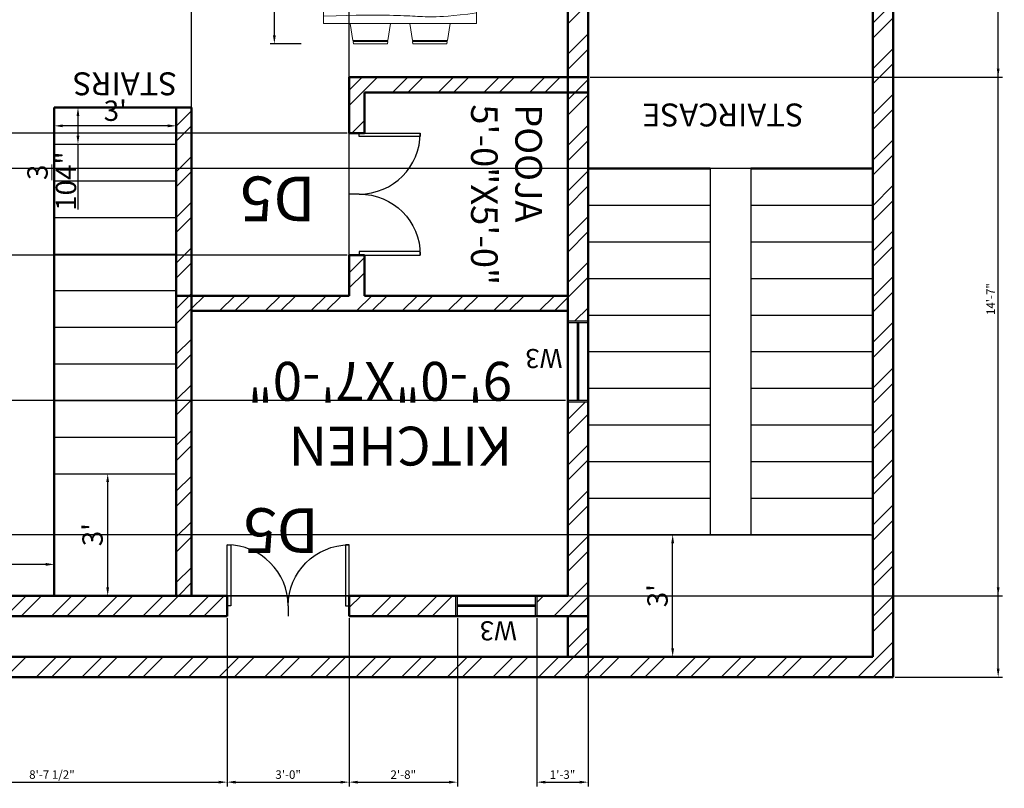
# Model space of a CAD drawing. Units: inches. Extents: x 244 to 2800, y 1060 to 1700.
# Tile 7 of 13: x 1735 to 2025, y 1060 to 1287. Entities that reach past the tile are written whole.
import ezdxf

# ---------------------------------------------------------------- set-up
doc = ezdxf.new("R2010")
doc.units = ezdxf.units.IN
for name, color, linetype, lineweight in [('A-ANNO-DIMS', 2, 'Continuous', 18), ('A-ANNO-TEXT', 1, 'Continuous', 18), ('A-DOOR', 5, 'Continuous', 25), ('A-FLOR-STRS', 6, 'Continuous', 25), ('A-FURN', 9, 'Continuous', 18), ('A-GLAZ', 3, 'Continuous', 25), ('A-WALL', 7, 'Continuous', 50), ('A-WALL-PATT', 8, 'Continuous', 13)]:
    doc.layers.add(name, color=color, linetype=linetype, lineweight=lineweight)
doc.styles.get("Standard").update_dxf_attribs({"font": 'arial.ttf'})
doc.dimstyles.new('ISO-25', dxfattribs={"dimtxt": 2.5, "dimasz": 2.5, "dimexe": 1.25, "dimexo": 0.625, "dimtad": 1, "dimlunit": 4, "dimtxsty": 'Standard', "dimcen": 2.5, "dimadec": 0, "dimazin": 0, "dimtfac": 1, "dimtmove": 0, "dimatfit": 3, "dimfxl": 1, "dimarcsym": 0})

# ---------------------------------------------------------------- blocks, each defined once
blk = doc.blocks.new('*U2')
for p, q in [((0, 0), (0, -5)), ((30, 0), (30, -5))]:
    blk.add_line(p, q)
blk.add_lwpolyline([(0, 0), (0, 30), (1.75, 30), (1.75, 0)], close=True)
blk.add_arc((0, 0), 30, 0, 90)
blk = doc.blocks.new('Dining Set - 36 x 72 in.')
for p, q in [((-22.2343, 26.00059), (-23.4847, 17.99762)), ((-22.2304, 26), (-5.7608, 26)), ((-22, 27.5), (-22.1562, 26.50042)), ((-5.8416, 26.5), (-22.1534, 26.5)), ((-22, 27.5), (-6, 27.5)), ((-5.8437, 26.49966), (-6, 27.5)), ((-4.5152, 17.99762), (-5.7655, 25.99926)), ((5.7657, 26.00059), (4.5153, 17.99762)), ((5.7696, 26), (22.2392, 26)), ((6, 27.5), (5.8438, 26.50042)), ((22.1584, 26.5), (5.8466, 26.5)), ((6, 27.5), (22, 27.5)), ((22.1563, 26.49966), (22, 27.5)), ((23.4848, 17.99762), (22.2345, 25.99926)), ((36, 18), (-36, 18)), ((-36, 18), (-36, -18)), ((36, -18), (36, 18)), ((-44.0006, 8.23428), (-35.9976, 9.48474)), ((44.0006, 8.23428), (35.9976, 9.48474)), ((-45.5, 8), (-44.5004, 8.15617)), ((-45.5, 8), (-45.5, -8)), ((-44.5, -8.15843), (-44.5, 8.15338)), ((-44, 8.23041), (-44, -8.23915)), ((44, 8.23041), (44, -8.23915)), ((44.5, -8.15843), (44.5, 8.15338)), ((45.5, 8), (44.5005, 8.15617)), ((45.5, 8), (45.5, -8)), ((-44.4997, -8.15631), (-45.5, -8)), ((-35.9976, -9.48476), (-43.9993, -8.2345)), ((35.9976, -9.48476), (43.9993, -8.2345)), ((44.4997, -8.15631), (45.5, -8)), ((-36, -18), (36, -18)), ((-22.2343, -26.0006), (-23.4847, -17.99762)), ((-4.5152, -17.99762), (-5.7655, -25.99928)), ((5.7657, -26.0006), (4.5153, -17.99762)), ((23.4848, -17.99762), (22.2345, -25.99928)), ((-22.2304, -26), (-5.7608, -26)), ((-22, -27.5), (-22.1562, -26.50044)), ((-5.8416, -26.5), (-22.1534, -26.5)), ((-22, -27.5), (-6, -27.5)), ((-5.8437, -26.49967), (-6, -27.5)), ((5.7696, -26), (22.2392, -26)), ((6, -27.5), (5.8438, -26.50044)), ((22.1584, -26.5), (5.8466, -26.5)), ((6, -27.5), (22, -27.5)), ((22.1563, -26.49967), (22, -27.5))]:
    blk.add_line(p, q)
for points in [[(-36, 15), (-31.1772, 14.97754), (-26.8079, 14.91406), (-22.8538, 14.81543), (-19.276, 14.6875), (-16.0362, 14.53613), (-13.0957, 14.36718), (-10.4159, 14.18652), (-7.9583, 14), (-5.6904, 13.81315), (-3.6035, 13.63021), (-1.6954, 13.45508), (0.0365, 13.29166), (1.5945, 13.14388), (2.9811, 13.01562), (4.1988, 12.9108), (5.25, 12.83333), (6.1393, 12.78613), (6.8802, 12.76823), (7.4883, 12.77767), (7.9792, 12.8125), (8.3685, 12.87077), (8.6719, 12.95052), (8.9049, 13.0498), (9.0833, 13.16666), (9.2205, 13.29899), (9.3216, 13.44401), (9.3895, 13.59879), (9.4271, 13.76041), (9.4373, 13.92594), (9.4232, 14.09245), (9.3875, 14.257), (9.3333, 14.41666), (9.2638, 14.56917), (9.1836, 14.71484), (9.0975, 14.85465), (9.0104, 14.98958), (8.9272, 15.1206), (8.8529, 15.2487), (8.7922, 15.37483), (8.75, 15.5), (8.7305, 15.62467), (8.7344, 15.74739), (8.7617, 15.86621), (8.8125, 15.97916), (8.8867, 16.08431), (8.9844, 16.17968), (9.1055, 16.26334), (9.25, 16.33333), (9.4189, 16.38802), (9.6172, 16.42708), (9.8506, 16.45052), (10.125, 16.45833), (10.4463, 16.45052), (10.8203, 16.42708), (11.2529, 16.38802), (11.75, 16.33333), (12.3184, 16.26318), (12.9694, 16.17838), (13.7151, 16.07991), (14.5677, 15.96875), (15.5395, 15.84586), (16.6426, 15.71224), (17.8893, 15.56884), (19.2917, 15.41666), (20.859, 15.25667), (22.5879, 15.08984), (24.4721, 14.91715), (26.5052, 14.73958), (28.6809, 14.5581), (30.9929, 14.3737), (33.4347, 14.18733), (36, 14)], [(-36, 10), (-28.9766, 10.14274), (-23.1725, 10.20442), (-18.4241, 10.19775), (-14.5677, 10.13541), (-11.4399, 10.03011), (-8.877, 9.89453), (-6.7154, 9.74137), (-4.7917, 9.58333), (-2.9698, 9.43082), (-1.2246, 9.28515), (0.4415, 9.14534), (2.026, 9.01041), (3.5266, 8.87939), (4.9408, 8.7513), (6.266, 8.62516), (7.5, 8.5), (8.6411, 8.37549), (9.6914, 8.2539), (10.6538, 8.13818), (11.5312, 8.03125), (12.3267, 7.93603), (13.043, 7.85547), (13.6831, 7.79248), (14.25, 7.75), (14.7471, 7.7303), (15.1797, 7.73307), (15.5537, 7.75732), (15.875, 7.80208), (16.1494, 7.86637), (16.3828, 7.94922), (16.5811, 8.04964), (16.75, 8.16666), (16.8944, 8.29915), (17.0143, 8.44531), (17.1089, 8.60319), (17.1771, 8.77083), (17.218, 8.94629), (17.2305, 9.1276), (17.2137, 9.31282), (17.1667, 9.5), (17.0895, 9.6875), (16.987, 9.875), (16.8649, 10.0625), (16.7292, 10.25), (16.5856, 10.4375), (16.4401, 10.625), (16.2985, 10.8125), (16.1667, 11), (16.05, 11.18733), (15.9518, 11.3737), (15.8752, 11.5581), (15.8229, 11.73958), (15.798, 11.91715), (15.8034, 12.08984), (15.842, 12.25667), (15.9167, 12.41666), (16.0295, 12.56836), (16.1784, 12.70833), (16.3605, 12.83268), (16.5729, 12.9375), (16.8127, 13.01888), (17.0768, 13.07291), (17.3625, 13.0957), (17.6667, 13.08333), (17.9894, 13.03312), (18.3418, 12.94726), (18.7382, 12.82918), (19.1927, 12.68229), (19.7195, 12.51001), (20.3327, 12.31575), (21.0465, 12.10294), (21.875, 11.875), (22.8357, 11.63354), (23.959, 11.37304), (25.2786, 11.08618), (26.8282, 10.76562), (28.6414, 10.40405), (30.752, 9.99414), (33.1936, 9.52856), (36, 9)], [(-36, 5.5), (-30.7157, 5.3348), (-26.069, 5.20963), (-21.9946, 5.11767), (-18.4271, 5.05208), (-15.3009, 5.00602), (-12.5508, 4.97265), (-10.1112, 4.94515), (-7.9167, 4.91666), (-5.909, 4.88167), (-4.0586, 4.83984), (-2.3429, 4.79215), (-0.7396, 4.73958), (0.7739, 4.6831), (2.22, 4.6237), (3.6213, 4.56233), (5, 4.5), (6.373, 4.43782), (7.7344, 4.3776), (9.0723, 4.32129), (10.375, 4.27083), (11.6309, 4.22819), (12.8281, 4.19531), (13.9551, 4.17415), (15, 4.16666), (15.954, 4.17448), (16.819, 4.19791), (17.6001, 4.23698), (18.3021, 4.29166), (18.9299, 4.36198), (19.4883, 4.44791), (19.9823, 4.54948), (20.4167, 4.66666), (20.7969, 4.79899), (21.1302, 4.94401), (21.4245, 5.09879), (21.6875, 5.26041), (21.9271, 5.42594), (22.1511, 5.59245), (22.3672, 5.757), (22.5834, 5.91666), (22.8065, 6.06868), (23.0404, 6.21093), (23.2879, 6.34147), (23.5521, 6.45833), (23.8358, 6.55957), (24.142, 6.64323), (24.4735, 6.70735), (24.8334, 6.75), (25.2235, 6.76969), (25.642, 6.76692), (26.0858, 6.74267), (26.5521, 6.69791), (27.0379, 6.63362), (27.5404, 6.55078), (28.0565, 6.45036), (28.5834, 6.33333), (29.1242, 6.19987), (29.7071, 6.04687), (30.3661, 5.87044), (31.1354, 5.66666), (32.0493, 5.43164), (33.142, 5.16146), (34.4475, 4.85221), (36, 4.5)], [(-36, -1), (-30.7915, -0.6591), (-26.0195, -0.38216), (-21.6519, -0.16284), (-17.6563, 0.00521), (-14.0005, 0.12833), (-10.6523, 0.21289), (-7.5796, 0.26522), (-4.75, 0.29166), (-2.134, 0.29793), (0.2878, 0.28711), (2.5317, 0.26163), (4.6146, 0.22396), (6.5529, 0.17651), (8.3633, 0.12174), (10.0623, 0.06209), (11.6667, 0), (13.1899, -0.06201), (14.6341, -0.1211), (15.9982, -0.17432), (17.2813, -0.21875), (18.4823, -0.25147), (19.6003, -0.26953), (20.6343, -0.27002), (21.5834, -0.25), (22.4481, -0.20768), (23.2357, -0.14584), (23.9549, -0.06836), (24.6146, 0.02083), (25.2235, 0.11784), (25.7904, 0.21875), (26.3241, 0.31966), (26.8334, 0.41666), (27.3265, 0.50618), (27.8099, 0.58593), (28.2894, 0.65397), (28.7709, 0.70833), (29.2601, 0.74707), (29.763, 0.76823), (30.2855, 0.76985), (30.8334, 0.75), (31.4088, 0.70784), (31.9994, 0.64713), (32.589, 0.57275), (33.1615, 0.48958), (33.7008, 0.4025), (34.1908, 0.3164), (34.6153, 0.23616), (34.9584, 0.16666), (35.2099, 0.11165), (35.3848, 0.07031), (35.504, 0.04069), (35.5886, 0.02083), (35.6594, 0.00879), (35.7377, 0.0026), (35.8442, 0.00032), (36, 0)], [(-36, -6.5), (-27.1843, -6.31267), (-20.084, -6.1263), (-14.469, -5.9419), (-10.1094, -5.76042), (-6.7752, -5.58285), (-4.2363, -5.41016), (-2.2629, -5.24333), (-0.625, -5.08334), (0.8708, -4.93099), (2.2715, -4.78646), (3.5872, -4.64974), (4.8281, -4.52084), (6.0046, -4.39974), (7.127, -4.28646), (8.2053, -4.18099), (9.25, -4.08334), (10.2705, -3.99382), (11.2734, -3.91407), (12.2647, -3.84603), (13.25, -3.79167), (14.2354, -3.75293), (15.2266, -3.73177), (16.2295, -3.73015), (17.25, -3.75), (18.2912, -3.79248), (19.3451, -3.85547), (20.4009, -3.93604), (21.4479, -4.03125), (22.4754, -4.13819), (23.4727, -4.25391), (24.4289, -4.37549), (25.3334, -4.5), (26.1785, -4.62492), (26.9694, -4.74935), (27.7145, -4.87281), (28.4219, -4.99479), (29.1, -5.11483), (29.7572, -5.23242), (30.4016, -5.34709), (31.0417, -5.45834), (31.6837, -5.56437), (32.3262, -5.65821), (32.9658, -5.73153), (33.599, -5.77604), (34.2224, -5.78345), (34.8327, -5.74545), (35.4264, -5.65373), (36, -5.5)], [(-36, -10), (-26.4022, -9.81299), (-18.4675, -9.62891), (-11.9839, -9.45069), (-6.7396, -9.28125), (-2.5226, -9.12354), (0.8789, -8.98047), (3.6769, -8.85498), (6.0833, -8.75), (8.2767, -8.66765), (10.3021, -8.60677), (12.1712, -8.56543), (13.8958, -8.54167), (15.4876, -8.53353), (16.9583, -8.53907), (18.3197, -8.55632), (19.5834, -8.58334), (20.7616, -8.61841), (21.8685, -8.66081), (22.9188, -8.71004), (23.9271, -8.76563), (24.9081, -8.82707), (25.8763, -8.89388), (26.8465, -8.96558), (27.8334, -9.04167), (28.8474, -9.12118), (29.8828, -9.20117), (30.93, -9.27824), (31.9792, -9.34896), (33.0205, -9.40991), (34.0443, -9.45768), (35.0407, -9.48885), (36, -9.5)], [(-36, -14.5), (-30.0881, -14.33513), (-25.0332, -14.21224), (-20.7312, -14.12647), (-17.0781, -14.07292), (-13.97, -14.04671), (-11.3027, -14.04297), (-8.9724, -14.05681), (-6.875, -14.08334), (-4.9224, -14.11833), (-3.0905, -14.16016), (-1.3709, -14.20785), (0.2448, -14.26042), (1.7647, -14.3169), (3.1973, -14.3763), (4.5507, -14.43767), (5.8333, -14.5), (7.0554, -14.5621), (8.235, -14.62175), (9.3922, -14.67652), (10.5469, -14.72396), (11.7192, -14.76164), (12.929, -14.78711), (14.1965, -14.79794), (15.5417, -14.79167), (16.9933, -14.76424), (18.6152, -14.70508), (20.4804, -14.60197), (22.6615, -14.44271), (25.2312, -14.21509), (28.2624, -13.9069), (31.8277, -13.50594), (36, -13)]]:
    blk.add_lwpolyline(points)
blk = doc.blocks.new('*D38')
at = {"layer": 'A-ANNO-DIMS', "color": 0, "lineweight": -2, "transparency": 16777216}
for p, q in [((1708.9, 1124.22), (1708.9, 1127.48)), ((1744.9, 1124.22), (1744.9, 1127.48)), ((1742.4, 1126.23), (1711.4, 1126.23))]:
    blk.add_line(p, q, dxfattribs=at)
at = {"layer": 'A-ANNO-DIMS', "color": 0, "transparency": 16777216}
for points in [[(1711.4, 1126.65), (1711.4, 1125.81), (1708.9, 1126.23)], [(1742.4, 1126.65), (1742.4, 1125.81), (1744.9, 1126.23)]]:
    blk.add_solid(points, dxfattribs=at)
at = {"layer": 'Defpoints', "color": 0, "transparency": 16777216}
for p in [(1708.9, 1126.23), (1708.9, 1123.59), (1744.9, 1123.59)]:
    blk.add_point(p, dxfattribs=at)
at = {"layer": 'A-ANNO-DIMS', "color": 0, "transparency": 16777216, "insert": (1726.9, 1129.92), "char_height": 6, "attachment_point": 5}
blk.add_mtext("3'", dxfattribs=at)
blk = doc.blocks.new('*D40')
at = {"layer": 'A-ANNO-DIMS', "color": 0, "lineweight": -2, "transparency": 16777216}
for p, q in [((1744.9, 1260.36), (1744.9, 1254.35)), ((1780.9, 1260.36), (1780.9, 1254.35)), ((1778.4, 1255.6), (1747.4, 1255.6))]:
    blk.add_line(p, q, dxfattribs=at)
at = {"layer": 'A-ANNO-DIMS', "color": 0, "transparency": 16777216}
for points in [[(1747.4, 1256.02), (1747.4, 1255.19), (1744.9, 1255.6)], [(1778.4, 1256.02), (1778.4, 1255.19), (1780.9, 1255.6)]]:
    blk.add_solid(points, dxfattribs=at)
at = {"layer": 'Defpoints', "color": 0, "transparency": 16777216}
for p in [(1744.9, 1260.99), (1780.9, 1260.99), (1744.9, 1255.6)]:
    blk.add_point(p, dxfattribs=at)
at = {"layer": 'A-ANNO-DIMS', "color": 0, "transparency": 16777216, "insert": (1762.9, 1259.29), "char_height": 6, "attachment_point": 5}
blk.add_mtext("3'", dxfattribs=at)
blk = doc.blocks.new('*D41')
at = {"layer": 'A-ANNO-DIMS', "color": 0, "lineweight": -2, "transparency": 16777216}
for p, q in [((1745.52, 1260.99), (1753.14, 1260.99)), ((1751.89, 1258.49), (1751.89, 1252.69)), ((1745.52, 1250.19), (1753.14, 1250.19)), ((1751.89, 1250.19), (1751.89, 1230.89))]:
    blk.add_line(p, q, dxfattribs=at)
at = {"layer": 'A-ANNO-DIMS', "color": 0, "transparency": 16777216}
for points in [[(1751.47, 1258.49), (1752.3, 1258.49), (1751.89, 1260.99)], [(1751.47, 1252.69), (1752.3, 1252.69), (1751.89, 1250.19)]]:
    blk.add_solid(points, dxfattribs=at)
at = {"layer": 'Defpoints', "color": 0, "transparency": 16777216}
for p in [(1744.9, 1260.99), (1744.9, 1250.19), (1751.89, 1250.19)]:
    blk.add_point(p, dxfattribs=at)
at = {"layer": 'A-ANNO-DIMS', "color": 0, "transparency": 16777216, "insert": (1744.15, 1239.29), "char_height": 6, "attachment_point": 5, "rotation": 90}
blk.add_mtext('10{\\H1x;\\S3/4;}"', dxfattribs=at)
blk = doc.blocks.new('*D42')
at = {"layer": 'A-ANNO-DIMS', "color": 0, "lineweight": -2, "transparency": 16777216}
for p, q in [((1752.51, 1152.99), (1761.91, 1152.99)), ((1760.66, 1119.49), (1760.66, 1150.49)), ((1752.51, 1116.99), (1761.91, 1116.99))]:
    blk.add_line(p, q, dxfattribs=at)
at = {"layer": 'A-ANNO-DIMS', "color": 0, "transparency": 16777216}
for points in [[(1760.24, 1150.49), (1761.07, 1150.49), (1760.66, 1152.99)], [(1760.24, 1119.49), (1761.07, 1119.49), (1760.66, 1116.99)]]:
    blk.add_solid(points, dxfattribs=at)
at = {"layer": 'Defpoints', "color": 0, "transparency": 16777216}
for p in [(1751.89, 1152.99), (1760.66, 1152.99), (1751.89, 1116.99)]:
    blk.add_point(p, dxfattribs=at)
at = {"layer": 'A-ANNO-DIMS', "color": 0, "transparency": 16777216, "insert": (1756.97, 1134.99), "char_height": 6, "attachment_point": 5, "rotation": 90}
blk.add_mtext("3'", dxfattribs=at)
blk = doc.blocks.new('*D43')
at = {"layer": 'A-ANNO-DIMS', "color": 0, "lineweight": -2, "transparency": 16777216}
for p, q in [((1952.09, 1134.99), (1926.1, 1134.99)), ((1927.35, 1101.49), (1927.35, 1132.49)), ((1952.09, 1098.99), (1926.1, 1098.99))]:
    blk.add_line(p, q, dxfattribs=at)
at = {"layer": 'A-ANNO-DIMS', "color": 0, "transparency": 16777216}
for points in [[(1926.94, 1132.49), (1927.77, 1132.49), (1927.35, 1134.99)], [(1926.94, 1101.49), (1927.77, 1101.49), (1927.35, 1098.99)]]:
    blk.add_solid(points, dxfattribs=at)
at = {"layer": 'Defpoints', "color": 0, "transparency": 16777216}
for p in [(1927.35, 1134.99), (1952.71, 1134.99), (1952.71, 1098.99)]:
    blk.add_point(p, dxfattribs=at)
at = {"layer": 'A-ANNO-DIMS', "color": 0, "transparency": 16777216, "insert": (1923.66, 1116.99), "char_height": 6, "attachment_point": 5, "rotation": 90}
blk.add_mtext("3'", dxfattribs=at)
blk = doc.blocks.new('WIN-24')
for p, q in [((0, 0), (0, 23.94)), ((0, 23.94), (6, 23.94)), ((6, 23.94), (6, 0)), ((6, 0), (0, 0))]:
    blk.add_line(p, q)
blk = doc.blocks.new('*D73')
at = {"layer": 'A-ANNO-DIMS', "color": 0, "lineweight": -2, "transparency": 16777216}
for p, q in [((1817.77, 1314.32), (1808.58, 1314.32)), ((1809.83, 1282.32), (1809.83, 1311.82)), ((1817.77, 1279.82), (1808.58, 1279.82))]:
    blk.add_line(p, q, dxfattribs=at)
at = {"layer": 'A-ANNO-DIMS', "color": 0, "transparency": 16777216}
for points in [[(1809.42, 1311.82), (1810.25, 1311.82), (1809.83, 1314.32)], [(1809.42, 1282.32), (1810.25, 1282.32), (1809.83, 1279.82)]]:
    blk.add_solid(points, dxfattribs=at)
at = {"layer": 'Defpoints', "color": 0, "transparency": 16777216}
for p in [(1809.83, 1314.32), (1818.4, 1314.32), (1818.4, 1279.82)]:
    blk.add_point(p, dxfattribs=at)
at = {"layer": 'A-ANNO-DIMS', "color": 0, "transparency": 16777216, "insert": (1807.92, 1297.07), "char_height": 2.5, "attachment_point": 5, "rotation": 90}
blk.add_mtext('2\'-10 1/2"', dxfattribs=at)
blk = doc.blocks.new('*D75')
at = {"layer": 'A-ANNO-DIMS', "color": 0, "lineweight": -2, "transparency": 16777216}
for p, q in [((1993.02, 1632.99), (2024.65, 1632.99)), ((2023.4, 1095.49), (2023.4, 1630.49)), ((1993.02, 1092.99), (2024.65, 1092.99))]:
    blk.add_line(p, q, dxfattribs=at)
at = {"layer": 'A-ANNO-DIMS', "color": 0, "transparency": 16777216}
for points in [[(2022.98, 1630.49), (2023.81, 1630.49), (2023.4, 1632.99)], [(2022.98, 1095.49), (2023.81, 1095.49), (2023.4, 1092.99)]]:
    blk.add_solid(points, dxfattribs=at)
at = {"layer": 'Defpoints', "color": 0, "transparency": 16777216}
for p in [(1992.4, 1632.99), (2023.4, 1632.99), (1992.4, 1092.99)]:
    blk.add_point(p, dxfattribs=at)
at = {"layer": 'A-ANNO-DIMS', "color": 0, "transparency": 16777216, "insert": (2021.49, 1362.99), "char_height": 2.5, "attachment_point": 5, "rotation": 90}
blk.add_mtext('45\'-0"', dxfattribs=at)
blk = doc.blocks.new('*D85')
at = {"layer": 'A-ANNO-DIMS', "color": 0, "lineweight": -2, "transparency": 16777216}
for p, q in [((1537.02, 1291.99), (2024.65, 1291.99)), ((2023.4, 1119.49), (2023.4, 1289.49)), ((1537.02, 1116.99), (2024.65, 1116.99))]:
    blk.add_line(p, q, dxfattribs=at)
at = {"layer": 'A-ANNO-DIMS', "color": 0, "transparency": 16777216}
for points in [[(2022.98, 1289.49), (2023.81, 1289.49), (2023.4, 1291.99)], [(2022.98, 1119.49), (2023.81, 1119.49), (2023.4, 1116.99)]]:
    blk.add_solid(points, dxfattribs=at)
at = {"layer": 'Defpoints', "color": 0, "transparency": 16777216}
for p in [(1536.4, 1291.99), (2023.4, 1291.99), (1536.4, 1116.99)]:
    blk.add_point(p, dxfattribs=at)
at = {"layer": 'A-ANNO-DIMS', "color": 0, "transparency": 16777216, "insert": (2021.52, 1204.49), "char_height": 2.5, "attachment_point": 5, "rotation": 90}
blk.add_mtext('14\'-7"', dxfattribs=at)
blk = doc.blocks.new('*D95')
at = {"layer": 'A-ANNO-DIMS', "color": 0, "lineweight": -2, "transparency": 16777216}
for p, q in [((1692.52, 1110.36), (1692.52, 1060.74)), ((1795.9, 1110.36), (1795.9, 1060.74)), ((1695.02, 1061.99), (1793.4, 1061.99))]:
    blk.add_line(p, q, dxfattribs=at)
at = {"layer": 'A-ANNO-DIMS', "color": 0, "transparency": 16777216}
for points in [[(1695.02, 1062.4), (1695.02, 1061.57), (1692.52, 1061.99)], [(1793.4, 1062.4), (1793.4, 1061.57), (1795.9, 1061.99)]]:
    blk.add_solid(points, dxfattribs=at)
at = {"layer": 'Defpoints', "color": 0, "transparency": 16777216}
for p in [(1692.52, 1110.99), (1795.9, 1110.99), (1795.9, 1061.99)]:
    blk.add_point(p, dxfattribs=at)
at = {"layer": 'A-ANNO-DIMS', "color": 0, "transparency": 16777216, "insert": (1744.21, 1063.9), "char_height": 2.5, "attachment_point": 5}
blk.add_mtext('8\'-7 1/2"', dxfattribs=at)
blk = doc.blocks.new('*D96')
at = {"layer": 'A-ANNO-DIMS', "color": 0, "lineweight": -2, "transparency": 16777216}
for p, q in [((1795.9, 1110.36), (1795.9, 1060.74)), ((1831.9, 1110.36), (1831.9, 1060.74)), ((1798.4, 1061.99), (1829.4, 1061.99))]:
    blk.add_line(p, q, dxfattribs=at)
at = {"layer": 'A-ANNO-DIMS', "color": 0, "transparency": 16777216}
for points in [[(1798.4, 1062.4), (1798.4, 1061.57), (1795.9, 1061.99)], [(1829.4, 1062.4), (1829.4, 1061.57), (1831.9, 1061.99)]]:
    blk.add_solid(points, dxfattribs=at)
at = {"layer": 'Defpoints', "color": 0, "transparency": 16777216}
for p in [(1795.9, 1110.99), (1831.9, 1110.99), (1831.9, 1061.99)]:
    blk.add_point(p, dxfattribs=at)
at = {"layer": 'A-ANNO-DIMS', "color": 0, "transparency": 16777216, "insert": (1813.9, 1063.89), "char_height": 2.5, "attachment_point": 5}
blk.add_mtext('3\'-0"', dxfattribs=at)
blk = doc.blocks.new('*D97')
at = {"layer": 'A-ANNO-DIMS', "color": 0, "lineweight": -2, "transparency": 16777216}
for p, q in [((1831.9, 1110.36), (1831.9, 1060.74)), ((1863.85, 1110.36), (1863.85, 1060.74)), ((1834.4, 1061.99), (1861.35, 1061.99))]:
    blk.add_line(p, q, dxfattribs=at)
at = {"layer": 'A-ANNO-DIMS', "color": 0, "transparency": 16777216}
for points in [[(1834.4, 1062.4), (1834.4, 1061.57), (1831.9, 1061.99)], [(1861.35, 1062.4), (1861.35, 1061.57), (1863.85, 1061.99)]]:
    blk.add_solid(points, dxfattribs=at)
at = {"layer": 'Defpoints', "color": 0, "transparency": 16777216}
for p in [(1831.9, 1110.99), (1863.85, 1110.99), (1863.85, 1061.99)]:
    blk.add_point(p, dxfattribs=at)
at = {"layer": 'A-ANNO-DIMS', "color": 0, "transparency": 16777216, "insert": (1847.87, 1063.89), "char_height": 2.5, "attachment_point": 5}
blk.add_mtext('2\'-8"', dxfattribs=at)
blk = doc.blocks.new('*D98')
at = {"layer": 'A-ANNO-DIMS', "color": 0, "lineweight": -2, "transparency": 16777216}
for p, q in [((1887.3, 1110.36), (1887.3, 1060.74)), ((1902.4, 1110.36), (1902.4, 1060.74)), ((1889.8, 1061.99), (1899.9, 1061.99))]:
    blk.add_line(p, q, dxfattribs=at)
at = {"layer": 'A-ANNO-DIMS', "color": 0, "transparency": 16777216}
for points in [[(1889.8, 1062.4), (1889.8, 1061.57), (1887.3, 1061.99)], [(1899.9, 1062.4), (1899.9, 1061.57), (1902.4, 1061.99)]]:
    blk.add_solid(points, dxfattribs=at)
at = {"layer": 'Defpoints', "color": 0, "transparency": 16777216}
for p in [(1887.3, 1110.99), (1902.4, 1110.99), (1902.4, 1061.99)]:
    blk.add_point(p, dxfattribs=at)
at = {"layer": 'A-ANNO-DIMS', "color": 0, "transparency": 16777216, "insert": (1894.85, 1063.89), "char_height": 2.5, "attachment_point": 5}
blk.add_mtext('1\'-3"', dxfattribs=at)
blk = doc.blocks.new('*D102')
at = {"layer": 'A-ANNO-DIMS', "color": 0, "lineweight": -2, "transparency": 16777216}
for p, q in [((1903.02, 1405.58), (2024.65, 1405.58)), ((2023.4, 1272.49), (2023.4, 1403.08)), ((1903.02, 1269.99), (2024.65, 1269.99))]:
    blk.add_line(p, q, dxfattribs=at)
at = {"layer": 'A-ANNO-DIMS', "color": 0, "transparency": 16777216}
for points in [[(2022.98, 1403.08), (2023.81, 1403.08), (2023.4, 1405.58)], [(2022.98, 1272.49), (2023.81, 1272.49), (2023.4, 1269.99)]]:
    blk.add_solid(points, dxfattribs=at)
at = {"layer": 'Defpoints', "color": 0, "transparency": 16777216}
for p in [(1902.4, 1405.58), (2023.4, 1405.58), (1902.4, 1269.99)]:
    blk.add_point(p, dxfattribs=at)
at = {"layer": 'A-ANNO-DIMS', "color": 0, "transparency": 16777216, "insert": (2021.48, 1337.78), "char_height": 2.5, "attachment_point": 5, "rotation": 90}
blk.add_mtext('11\'-3 1/2"', dxfattribs=at)
blk = doc.blocks.new('*D103')
at = {"layer": 'A-ANNO-DIMS', "color": 0, "lineweight": -2, "transparency": 16777216}
for p, q in [((1985.77, 1242.99), (1480.15, 1242.99)), ((1481.4, 1137.49), (1481.4, 1240.49)), ((1985.77, 1134.99), (1480.15, 1134.99))]:
    blk.add_line(p, q, dxfattribs=at)
at = {"layer": 'A-ANNO-DIMS', "color": 0, "transparency": 16777216}
for points in [[(1480.98, 1240.49), (1481.81, 1240.49), (1481.4, 1242.99)], [(1480.98, 1137.49), (1481.81, 1137.49), (1481.4, 1134.99)]]:
    blk.add_solid(points, dxfattribs=at)
at = {"layer": 'Defpoints', "color": 0, "transparency": 16777216}
for p in [(1481.4, 1242.99), (1986.4, 1242.99), (1986.4, 1134.99)]:
    blk.add_point(p, dxfattribs=at)
at = {"layer": 'A-ANNO-DIMS', "color": 0, "transparency": 16777216, "insert": (1479.49, 1188.99), "char_height": 2.5, "attachment_point": 5, "rotation": 90}
blk.add_mtext('9\'-0"', dxfattribs=at)
blk = doc.blocks.new('*D104')
at = {"layer": 'A-ANNO-DIMS', "color": 0, "lineweight": -2, "transparency": 16777216}
for p, q in [((1785.4, 1201.61), (1785.4, 1665.24)), ((1831.9, 1206.11), (1831.9, 1665.24)), ((1787.9, 1663.99), (1829.4, 1663.99))]:
    blk.add_line(p, q, dxfattribs=at)
at = {"layer": 'A-ANNO-DIMS', "color": 0, "transparency": 16777216}
for points in [[(1787.9, 1664.4), (1787.9, 1663.57), (1785.4, 1663.99)], [(1829.4, 1664.4), (1829.4, 1663.57), (1831.9, 1663.99)]]:
    blk.add_solid(points, dxfattribs=at)
at = {"layer": 'Defpoints', "color": 0, "transparency": 16777216}
for p in [(1831.9, 1663.99), (1831.9, 1205.49), (1785.4, 1200.99)]:
    blk.add_point(p, dxfattribs=at)
at = {"layer": 'A-ANNO-DIMS', "color": 0, "transparency": 16777216, "insert": (1808.65, 1665.9), "char_height": 2.5, "attachment_point": 5}
blk.add_mtext('3\'-10 1/2"', dxfattribs=at)
blk = doc.blocks.new('*D105')
at = {"layer": 'A-ANNO-DIMS', "color": 0, "lineweight": -2, "transparency": 16777216}
for p, q in [((1831.27, 1253.49), (1480.15, 1253.49)), ((1481.4, 1219.99), (1481.4, 1250.99)), ((1831.27, 1217.49), (1480.15, 1217.49))]:
    blk.add_line(p, q, dxfattribs=at)
at = {"layer": 'A-ANNO-DIMS', "color": 0, "transparency": 16777216}
for points in [[(1480.98, 1250.99), (1481.81, 1250.99), (1481.4, 1253.49)], [(1480.98, 1219.99), (1481.81, 1219.99), (1481.4, 1217.49)]]:
    blk.add_solid(points, dxfattribs=at)
at = {"layer": 'Defpoints', "color": 0, "transparency": 16777216}
for p in [(1481.4, 1253.49), (1831.9, 1253.49), (1831.9, 1217.49)]:
    blk.add_point(p, dxfattribs=at)
at = {"layer": 'A-ANNO-DIMS', "color": 0, "transparency": 16777216, "insert": (1479.49, 1235.49), "char_height": 2.5, "attachment_point": 5, "rotation": 90}
blk.add_mtext('3\'-0"', dxfattribs=at)
blk = doc.blocks.new('*D106')
at = {"layer": 'A-ANNO-DIMS', "color": 0, "lineweight": -2, "transparency": 16777216}
for p, q in [((1895.77, 1174.6), (1480.15, 1174.6)), ((1481.4, 1119.49), (1481.4, 1172.1)), ((1895.77, 1116.99), (1480.15, 1116.99))]:
    blk.add_line(p, q, dxfattribs=at)
at = {"layer": 'A-ANNO-DIMS', "color": 0, "transparency": 16777216}
for points in [[(1480.98, 1172.1), (1481.81, 1172.1), (1481.4, 1174.6)], [(1480.98, 1119.49), (1481.81, 1119.49), (1481.4, 1116.99)]]:
    blk.add_solid(points, dxfattribs=at)
at = {"layer": 'Defpoints', "color": 0, "transparency": 16777216}
for p in [(1481.4, 1174.6), (1896.4, 1174.6), (1896.4, 1116.99)]:
    blk.add_point(p, dxfattribs=at)
at = {"layer": 'A-ANNO-DIMS', "color": 0, "transparency": 16777216, "insert": (1479.48, 1145.79), "char_height": 2.5, "attachment_point": 5, "rotation": 90}
blk.add_mtext('4\'-9 1/2"', dxfattribs=at)

msp = doc.modelspace()

# ---------------------------------------------------------------- hatches: boundary and pattern name
at = {"layer": 'A-WALL-PATT'}
h = msp.add_hatch(dxfattribs=at)
h.set_pattern_fill('ANSI32', color=256)
h.paths.add_polyline_path([(1992.396, 1092.986), (1992.396, 1632.986), (1512.396, 1632.986), (1512.396, 1092.986)])
h.paths.add_polyline_path([(1518.396, 1098.986), (1518.396, 1626.986), (1986.396, 1626.986), (1986.396, 1098.986), (1902.396, 1098.986)], flags=16)
h.paths.add_polyline_path([(1795.896, 1110.986), (1530.396, 1110.986), (1530.396, 1551.986), (1521.7, 1551.986), (1521.7, 1623.986), (1605.7, 1623.986), (1605.7, 1551.986), (1781.396, 1551.986), (1781.396, 1545.986), (1708.896, 1545.986), (1708.896, 1532.64), (1704.396, 1532.64), (1704.396, 1545.986), (1536.396, 1545.986), (1536.396, 1372.986), (1671.396, 1372.986), (1671.396, 1368.486), (1621.896, 1368.486), (1621.896, 1296.486), (1704.396, 1296.486), (1704.396, 1368.486), (1701.396, 1368.486), (1701.396, 1372.986), (1704.396, 1372.986), (1704.396, 1490.64), (1708.896, 1490.64), (1708.896, 1288.986), (1704.396, 1288.986), (1704.396, 1291.986), (1569.396, 1291.986), (1569.396, 1296.486), (1618.896, 1296.486), (1618.896, 1368.486), (1536.396, 1368.486), (1536.396, 1296.486), (1539.396, 1296.486), (1539.396, 1291.986), (1536.396, 1291.986), (1536.396, 1116.986), (1704.396, 1116.986), (1704.396, 1246.986), (1708.896, 1246.986), (1708.896, 1116.986), (1744.896, 1116.986), (1744.896, 1260.986), (1780.896, 1260.986), (1785.396, 1260.986), (1785.396, 1205.486), (1831.896, 1205.486), (1831.896, 1217.486), (1836.396, 1217.486), (1836.396, 1205.486), (1896.396, 1205.486), (1896.396, 1265.486), (1836.396, 1265.486), (1836.396, 1253.486), (1831.896, 1253.486), (1831.896, 1269.986), (1896.396, 1269.986), (1896.396, 1472.64), (1902.396, 1472.64), (1902.396, 1242.986), (1938.396, 1242.986), (1938.396, 1134.986), (1950.396, 1134.986), (1950.396, 1242.986), (1986.396, 1242.986), (1986.396, 1134.986), (1902.396, 1134.986), (1902.396, 1110.986), (1831.896, 1110.986), (1831.896, 1116.986), (1896.396, 1116.986), (1896.396, 1200.986), (1785.396, 1200.986), (1785.396, 1116.986), (1795.896, 1116.986)], flags=0)
h.paths.add_polyline_path([(1780.896, 1116.986), (1744.896, 1116.986), (1744.896, 1260.986), (1780.896, 1260.986)], flags=0)
h.paths.add_polyline_path([(1863.351, 1110.986), (1863.351, 1116.986), (1887.296, 1116.986), (1887.296, 1110.986)], flags=0)
h.paths.add_polyline_path([(1863.851, 1114.186), (1886.796, 1114.186), (1886.796, 1113.786), (1863.851, 1113.786)], flags=0)
h.paths.add_polyline_path([(1896.396, 1174.102), (1896.396, 1198.047), (1902.396, 1198.047), (1902.396, 1174.102)], flags=0)
h.paths.add_polyline_path([(1902.396, 1174.602), (1899.196, 1174.602), (1899.196, 1197.547), (1902.396, 1197.547)], flags=0)
h.paths.add_polyline_path([(1692.519, 1110.986), (1656.574, 1110.986), (1656.574, 1116.986), (1692.519, 1116.986)], flags=0)
h.paths.add_polyline_path([(1819.776, 1376.187), (1819.776, 1410.382, -0.249194), (1838.546, 1410.382), (1838.546, 1376.187, -0.249194)], flags=0)
h.paths.add_polyline_path([(1536.396, 1250.972), (1530.396, 1250.972), (1530.396, 1286.917), (1536.396, 1286.917)], flags=0)
h.paths.add_polyline_path([(1896.396, 1405.581), (1896.396, 1453.526), (1902.396, 1453.526), (1902.396, 1405.581)], flags=0)
h.paths.add_polyline_path([(1536.396, 1322.935), (1530.396, 1322.935), (1530.396, 1346.88), (1536.396, 1346.88)], flags=0)
h.paths.add_polyline_path([(1533.196, 1323.435), (1533.196, 1346.38), (1533.596, 1346.38), (1533.596, 1323.435)], flags=0)
h.paths.add_polyline_path([(1896.396, 1545.986), (1841.396, 1545.986), (1841.396, 1551.986), (1902.396, 1551.986), (1902.396, 1532.64), (1896.396, 1532.64)], flags=0)
h.paths.add_polyline_path([(1756.808, 1545.986), (1732.863, 1545.986), (1732.863, 1551.986), (1756.808, 1551.986)], flags=0)
h.paths.add_polyline_path([(1756.308, 1548.786), (1733.363, 1548.786), (1733.363, 1551.986), (1756.308, 1551.986)], flags=0)
h.paths.add_polyline_path([(1673.743, 1545.986), (1637.798, 1545.986), (1637.798, 1551.986), (1673.743, 1551.986)], flags=0)
h.paths.add_polyline_path([(1536.396, 1503.969), (1530.396, 1503.969), (1530.396, 1539.914), (1536.396, 1539.914)], flags=0)
h.paths.add_polyline_path([(1896.341, 1192.868), (1881.737, 1192.868), (1881.737, 1181.273), (1896.341, 1181.273)], flags=8)
h.paths.add_polyline_path([(1882.893, 1112.542), (1868.29, 1112.542), (1868.29, 1100.947), (1882.893, 1100.947)], flags=8)
h.paths.add_polyline_path([(1531.898, 1340.208), (1517.295, 1340.208), (1517.295, 1328.613), (1531.898, 1328.613)], flags=24)
h.paths.add_polyline_path([(1662.207, 1564.332), (1647.603, 1564.332), (1647.603, 1552.737), (1662.207, 1552.737)], flags=8)
h.paths.add_polyline_path([(1750.605, 1565.018), (1736.001, 1565.018), (1736.001, 1553.424), (1750.605, 1553.424)], flags=8)
h.paths.add_polyline_path([(1919.351, 1440.326), (1904.748, 1440.326), (1904.748, 1428.731), (1919.351, 1428.731)], flags=8)
h.paths.add_polyline_path([(1827.662, 1149.994), (1797.512, 1149.994), (1797.512, 1122.813), (1827.662, 1122.813)], flags=8)
h.paths.add_polyline_path([(1826.683, 1247.85), (1796.533, 1247.85), (1796.533, 1220.668), (1826.683, 1220.668)], flags=8)
h.paths.add_polyline_path([(1713.043, 1285.137), (1682.893, 1285.137), (1682.893, 1257.956), (1713.043, 1257.956)], flags=8)
h.paths.add_polyline_path([(1567.301, 1310.129), (1537.151, 1310.129), (1537.151, 1282.948), (1567.301, 1282.948)], flags=8)
h.paths.add_polyline_path([(1699.655, 1386.046), (1669.505, 1386.046), (1669.505, 1358.865), (1699.655, 1358.865)], flags=8)
h.paths.add_polyline_path([(1716.254, 1527.375), (1686.103, 1527.375), (1686.103, 1500.194), (1716.254, 1500.194)], flags=8)
h.paths.add_polyline_path([(1822.088, 1577.207), (1791.938, 1577.207), (1791.938, 1550.026), (1822.088, 1550.026)], flags=8)
h.paths.add_polyline_path([(1931.716, 1518.23), (1901.565, 1518.23), (1901.565, 1491.049), (1931.716, 1491.049)], flags=8)
h.paths.add_polyline_path([(1636.272, 1573.477), (1636.272, 1615.869), (1613.819, 1615.869), (1613.819, 1573.477)], flags=8)
h.paths.add_polyline_path([(1968.141, 1266.003), (1911.144, 1266.003), (1911.144, 1252.05), (1968.141, 1252.05)], flags=8)
h.paths.add_polyline_path([(1783.26, 1275.202), (1745.711, 1275.202), (1745.711, 1261.249), (1783.26, 1261.249)], flags=8)
h.paths.add_polyline_path([(1753.522, 1456.095), (1753.522, 1338.024), (1798.876, 1338.024), (1798.876, 1456.095)], flags=8)
h.paths.add_polyline_path([(1884.04, 1192.467), (1803.345, 1192.467), (1803.345, 1149.693), (1884.04, 1149.693)], flags=8)
h.paths.add_polyline_path([(1863.426, 1264.753), (1863.426, 1209.557), (1892.661, 1209.557), (1892.661, 1264.753)], flags=8)
h.paths.add_polyline_path([(1594.411, 1361.178), (1536.688, 1361.178), (1536.688, 1330.387), (1594.411, 1330.387)], flags=8)
h.paths.add_polyline_path([(1695.984, 1342.402), (1638.262, 1342.402), (1638.262, 1311.611), (1695.984, 1311.611)], flags=8)
h.paths.add_polyline_path([(1654.435, 1540.65), (1537.752, 1540.65), (1537.752, 1489.721), (1654.435, 1489.721)], flags=8)
h.paths.add_polyline_path([(1658.864, 1271.272), (1542.182, 1271.272), (1542.182, 1220.343), (1658.864, 1220.343)], flags=8)
h = msp.add_hatch(dxfattribs=at)
h.set_pattern_fill('ANSI32', color=256)
h.paths.add_polyline_path([(1902.396, 1405.581), (1896.396, 1405.581), (1896.396, 1269.986), (1902.396, 1269.986)])
h = msp.add_hatch(dxfattribs=at)
h.set_pattern_fill('ANSI32', color=256)
h.paths.add_polyline_path([(1896.396, 1269.986), (1831.896, 1269.986), (1831.896, 1253.486), (1834.896, 1253.486), (1836.396, 1253.486), (1836.396, 1265.486), (1896.396, 1265.486)])
h = msp.add_hatch(dxfattribs=at)
h.set_pattern_fill('ANSI32', color=256)
h.paths.add_polyline_path([(1902.396, 1269.986), (1896.396, 1269.986), (1896.396, 1265.486), (1902.396, 1265.486)])
h = msp.add_hatch(dxfattribs=at)
h.set_pattern_fill('ANSI32', color=256)
h.paths.add_polyline_path([(1902.396, 1265.486), (1896.396, 1265.486), (1896.396, 1198.047), (1902.396, 1198.047)])
h = msp.add_hatch(dxfattribs=at)
h.set_pattern_fill('ANSI32', color=256)
h.paths.add_polyline_path([(1785.396, 1260.986), (1780.896, 1260.986), (1780.896, 1205.486), (1785.396, 1205.486)])
h = msp.add_hatch(dxfattribs=at)
h.set_pattern_fill('ANSI32', color=256)
h.paths.add_polyline_path([(1896.396, 1205.486), (1836.396, 1205.486), (1836.396, 1217.486), (1834.896, 1217.486), (1831.896, 1217.486), (1831.896, 1205.486), (1785.396, 1205.486), (1785.396, 1200.986), (1896.396, 1200.986)])
h = msp.add_hatch(dxfattribs=at)
h.set_pattern_fill('ANSI32', color=256)
h.paths.add_polyline_path([(1785.396, 1205.486), (1780.896, 1205.486), (1780.896, 1116.986), (1785.396, 1116.986)])
h = msp.add_hatch(dxfattribs=at)
h.set_pattern_fill('ANSI32', color=256)
h.paths.add_polyline_path([(1902.396, 1174.102), (1896.396, 1174.102), (1896.396, 1116.986), (1887.296, 1116.986), (1887.296, 1110.986), (1902.396, 1110.986)])
h = msp.add_hatch(dxfattribs=at)
h.set_pattern_fill('ANSI32', color=256)
h.paths.add_polyline_path([(1795.896, 1116.986), (1692.519, 1116.986), (1692.519, 1110.986), (1795.896, 1110.986), (1795.896, 1113.986)])
h = msp.add_hatch(dxfattribs=at)
h.set_pattern_fill('ANSI32', color=256)
h.paths.add_polyline_path([(1863.351, 1116.986), (1831.896, 1116.986), (1831.896, 1113.986), (1831.896, 1110.986), (1863.351, 1110.986)])
h = msp.add_hatch(dxfattribs=at)
h.set_pattern_fill('ANSI32', color=256)
h.paths.add_polyline_path([(1902.396, 1110.986), (1896.396, 1110.986), (1896.396, 1098.986), (1902.396, 1098.986)])

# ---------------------------------------------------------------- linework, layer by layer
at = {"layer": 'A-FLOR-STRS'}
for p, q in [((1744.896, 1116.986), (1744.896, 1260.986)), ((1744.896, 1260.986), (1780.896, 1260.986)), ((1744.896, 1260.986), (1780.896, 1260.986)), ((1744.896, 1250.186), (1780.896, 1250.186)), ((1902.396, 1242.986), (1938.396, 1242.986)), ((1902.396, 1242.986), (1902.396, 1098.986)), ((1902.396, 1242.986), (1938.396, 1242.986)), ((1938.396, 1242.986), (1938.396, 1134.986)), ((1950.396, 1242.986), (1986.396, 1242.986)), ((1950.396, 1242.986), (1950.396, 1134.986)), ((1950.396, 1242.986), (1986.396, 1242.986)), ((1986.396, 1242.986), (1986.396, 1098.986)), ((1744.896, 1239.386), (1780.896, 1239.386)), ((1902.396, 1232.186), (1938.396, 1232.186)), ((1950.396, 1232.186), (1986.396, 1232.186)), ((1744.896, 1228.586), (1780.896, 1228.586)), ((1902.396, 1221.386), (1938.396, 1221.386)), ((1950.396, 1221.386), (1986.396, 1221.386)), ((1744.896, 1217.786), (1780.896, 1217.786)), ((1902.396, 1210.586), (1938.396, 1210.586)), ((1950.396, 1210.586), (1986.396, 1210.586)), ((1744.896, 1206.986), (1780.896, 1206.986)), ((1902.396, 1199.786), (1938.396, 1199.786)), ((1950.396, 1199.786), (1986.396, 1199.786)), ((1744.896, 1196.186), (1780.896, 1196.186)), ((1902.396, 1188.986), (1938.396, 1188.986)), ((1950.396, 1188.986), (1986.396, 1188.986)), ((1744.896, 1185.386), (1780.896, 1185.386)), ((1902.396, 1178.186), (1938.396, 1178.186)), ((1950.396, 1178.186), (1986.396, 1178.186)), ((1744.896, 1174.586), (1780.896, 1174.586)), ((1902.396, 1167.386), (1938.396, 1167.386)), ((1950.396, 1167.386), (1986.396, 1167.386)), ((1744.896, 1163.786), (1780.896, 1163.786)), ((1902.396, 1156.586), (1938.396, 1156.586)), ((1950.396, 1156.586), (1986.396, 1156.586)), ((1744.896, 1152.986), (1780.896, 1152.986)), ((1902.396, 1145.786), (1938.396, 1145.786)), ((1950.396, 1145.786), (1986.396, 1145.786)), ((1902.396, 1134.986), (1986.396, 1134.986)), ((1744.896, 1116.986), (1780.896, 1116.986)), ((1902.396, 1098.986), (1986.396, 1098.986))]:
    msp.add_line(p, q, dxfattribs=at)
at = {"layer": 'A-GLAZ'}
for p, q in [((1896.396, 1197.547), (1902.396, 1197.547)), ((1899.196, 1197.547), (1899.196, 1174.602)), ((1899.596, 1197.547), (1899.596, 1174.602)), ((1902.396, 1174.602), (1896.396, 1174.602)), ((1863.851, 1110.986), (1863.851, 1116.986)), ((1886.796, 1116.986), (1886.796, 1110.986)), ((1886.796, 1114.186), (1863.851, 1114.186)), ((1886.796, 1113.786), (1863.851, 1113.786))]:
    msp.add_line(p, q, dxfattribs=at)
at = {"layer": 'A-WALL'}
for p, q in [((1992.396, 1092.986), (1992.396, 1632.986)), ((1986.396, 1098.986), (1986.396, 1626.986)), ((1896.396, 1116.986), (1896.396, 1472.64)), ((1902.396, 1098.986), (1902.396, 1472.64)), ((1831.896, 1269.986), (1902.396, 1269.986)), ((1831.896, 1253.486), (1831.896, 1269.986)), ((1836.396, 1265.486), (1902.396, 1265.486)), ((1836.396, 1265.486), (1836.396, 1253.486)), ((1836.396, 1253.486), (1836.396, 1265.486)), ((1744.896, 1260.986), (1744.896, 1116.986)), ((1744.896, 1260.986), (1785.396, 1260.986)), ((1780.896, 1260.986), (1780.896, 1116.986)), ((1785.396, 1260.986), (1785.396, 1116.986)), ((1836.396, 1253.486), (1831.896, 1253.486)), ((1902.396, 1242.986), (1938.396, 1242.986)), ((1950.396, 1242.986), (1986.396, 1242.986)), ((1831.896, 1205.486), (1831.896, 1217.486)), ((1831.896, 1217.486), (1836.396, 1217.486)), ((1836.396, 1205.486), (1836.396, 1217.486)), ((1780.896, 1205.486), (1831.896, 1205.486)), ((1836.396, 1205.486), (1896.396, 1205.486)), ((1785.396, 1200.986), (1896.396, 1200.986)), ((1536.396, 1116.986), (1795.896, 1116.986)), ((1785.396, 1116.986), (1795.896, 1116.986)), ((1795.896, 1116.986), (1795.896, 1110.986)), ((1831.896, 1110.986), (1831.896, 1116.986)), ((1831.896, 1116.986), (1896.396, 1116.986)), ((1530.396, 1110.986), (1795.896, 1110.986)), ((1831.896, 1110.986), (1902.396, 1110.986)), ((1896.396, 1098.986), (1896.396, 1110.986)), ((1518.396, 1098.986), (1986.396, 1098.986)), ((1512.396, 1092.986), (1992.396, 1092.986))]:
    msp.add_line(p, q, dxfattribs=at)

# ---------------------------------------------------------------- block references
at = {"layer": 'A-DOOR', "yscale": 0.6000000000000038, "zscale": 0.6000000000000038, "rotation": 270}
for p, xscale in [((1834.896, 1253.486), 0.6000000000000038), ((1834.896, 1217.486), -0.6000000000000038)]:
    msp.add_blockref('*U2', p, dxfattribs=dict(at, xscale=xscale))
at = {"layer": 'A-DOOR', "yscale": 0.6000000000000038, "zscale": 0.6000000000000038}
for p, xscale in [((1795.896, 1113.986), 0.6000000000000038), ((1831.896, 1113.986), -0.6000000000000038)]:
    msp.add_blockref('*U2', p, dxfattribs=dict(at, xscale=xscale))
at = {"layer": 'A-FURN', "xscale": 0.627265132509438, "yscale": 0.627265132509438, "zscale": 0.627265132509438}
msp.add_blockref('Dining Set - 36 x 72 in.', (1846.937, 1297.066), dxfattribs=at)
at = {"layer": 'A-GLAZ'}
msp.add_blockref('WIN-24', (1896.396, 1174.102), dxfattribs=at)
at = {"layer": 'A-GLAZ', "rotation": 90.00000000000156}
msp.add_blockref('WIN-24', (1887.296, 1110.986), dxfattribs=at)

# ---------------------------------------------------------------- texts
at = {"layer": 'A-ANNO-TEXT', "attachment_point": 1}
for s, width, gutter_width, insert, char_height, rotation in [('STAIRS', 2.71935, 33.854, (1781.142, 1264.618), 6.7708, 180), ('POOJA\\P5\'-0"X5\'-0"', 2.68471, 39.174, (1888.768, 1261.95), 7.83479, 270), ('STAIRCASE', 2.71935, 33.854, (1966.023, 1255.419), 6.7708, 180), ('D5', 20.58737, 65.951, (1821.964, 1227.457), 13.1902, 180), ('W3', 2.91536, 28.132, (1894.838, 1184.146), 5.6265, 180), ('KITCHEN\\P9\'-0"X7\'-0"', 18.53908, 57.316, (1880.002, 1155.397), 11.46316, 180), ('D5', 20.58737, 65.951, (1822.943, 1129.602), 13.1902, 180), ('W3', 2.91536, 28.132, (1881.391, 1103.82), 5.6265, 180)]:
    msp.add_mtext_dynamic_manual_height_columns(s, width=width, gutter_width=gutter_width, heights=[0], dxfattribs=dict(at, insert=insert, char_height=char_height, rotation=rotation))

# ---------------------------------------------------------------- dimensions: what is measured, and where the dimension line sits
at = {"layer": 'A-ANNO-DIMS'}
for base, p1, p2, override, picture, middle in [((1831.896, 1663.986), (1785.396, 1200.986), (1831.896, 1205.486), {"dimdec": 1, "dimlfac": 1, "dimrnd": 0, "dimzin": 1, "dimdsep": 46, "dimlunit": 4, "dimfrac": 2}, '*D104', (1808.646, 1665.905)), ((1744.896, 1255.602), (1780.896, 1260.986), (1744.896, 1260.986), {"dimtxt": 6, "dimclrd": 0, "dimclre": 0, "dimclrt": 0}, '*D40', (1762.896, 1259.292)), ((1708.896, 1126.23), (1744.896, 1123.591), (1708.896, 1123.591), {"dimtxt": 6, "dimclrd": 0, "dimclre": 0, "dimclrt": 0}, '*D38', (1726.896, 1129.921)), ((1795.896, 1061.986), (1692.519, 1110.986), (1795.896, 1110.986), {"dimdec": 1, "dimlfac": 1, "dimrnd": 0, "dimzin": 1, "dimdsep": 46, "dimlunit": 4, "dimfrac": 2}, '*D95', (1744.208, 1063.904)), ((1831.896, 1061.986), (1795.896, 1110.986), (1831.896, 1110.986), {"dimdec": 1, "dimlfac": 1, "dimrnd": 0, "dimzin": 1, "dimdsep": 46, "dimlunit": 4, "dimfrac": 2}, '*D96', (1813.896, 1063.888)), ((1863.851, 1061.986), (1831.896, 1110.986), (1863.851, 1110.986), {"dimdec": 1, "dimlfac": 1, "dimrnd": 0, "dimzin": 1, "dimdsep": 46, "dimlunit": 4, "dimfrac": 2}, '*D97', (1847.873, 1063.888)), ((1902.396, 1061.986), (1887.296, 1110.986), (1902.396, 1110.986), {"dimdec": 1, "dimlfac": 1, "dimrnd": 0, "dimzin": 1, "dimdsep": 46, "dimlunit": 4, "dimfrac": 2}, '*D98', (1894.846, 1063.888))]:
    dim = msp.add_linear_dim(base=base, p1=p1, p2=p2, dimstyle='ISO-25', override=override, dxfattribs=at)
    dim.commit()
    dim.dimension.update_dxf_attribs({"geometry": picture, "text_midpoint": middle})
for base, p1, p2, override, picture, middle in [((2023.396, 1632.986), (1992.396, 1092.986), (1992.396, 1632.986), {"dimdec": 1, "dimlfac": 1, "dimrnd": 0, "dimzin": 1, "dimdsep": 46, "dimlunit": 4, "dimfrac": 2}, '*D75', (2021.494, 1362.986)), ((2023.396, 1405.581), (1902.396, 1269.986), (1902.396, 1405.581), {"dimdec": 1, "dimlfac": 1, "dimrnd": 0, "dimzin": 1, "dimdsep": 46, "dimlunit": 4, "dimfrac": 2}, '*D102', (2021.477, 1337.784)), ((1809.834, 1314.316), (1818.397, 1279.816), (1818.397, 1314.316), {"dimdec": 1, "dimrnd": 0, "dimzin": 1, "dimlunit": 4, "dimfrac": 2}, '*D73', (1807.917, 1297.066)), ((2023.396, 1291.986), (1536.396, 1116.986), (1536.396, 1291.986), {"dimdec": 1, "dimlfac": 1, "dimrnd": 0, "dimzin": 1, "dimdsep": 46, "dimlunit": 4, "dimfrac": 2}, '*D85', (2021.516, 1204.486)), ((1751.887, 1250.186), (1744.896, 1260.986), (1744.896, 1250.186), {"dimtxt": 6, "dimclrd": 0, "dimclre": 0, "dimclrt": 0}, '*D41', (1744.146, 1239.289)), ((1481.396, 1253.486), (1831.896, 1217.486), (1831.896, 1253.486), {"dimdec": 1, "dimlfac": 1, "dimrnd": 0, "dimzin": 1, "dimdsep": 46, "dimlunit": 4, "dimfrac": 2}, '*D105', (1479.493, 1235.486)), ((1481.396, 1242.986), (1986.396, 1134.986), (1986.396, 1242.986), {"dimdec": 1, "dimlfac": 1, "dimrnd": 0, "dimzin": 1, "dimdsep": 46, "dimlunit": 4, "dimfrac": 2}, '*D103', (1479.494, 1188.986)), ((1481.396, 1174.602), (1896.396, 1116.986), (1896.396, 1174.602), {"dimdec": 1, "dimlfac": 1, "dimrnd": 0, "dimzin": 1, "dimdsep": 46, "dimlunit": 4, "dimfrac": 2}, '*D106', (1479.478, 1145.794)), ((1760.656, 1152.986), (1751.887, 1116.986), (1751.887, 1152.986), {"dimtxt": 6, "dimclrd": 0, "dimclre": 0, "dimclrt": 0}, '*D42', (1756.966, 1134.986)), ((1927.352, 1134.986), (1952.711, 1098.986), (1952.711, 1134.986), {"dimtxt": 6, "dimclrd": 0, "dimclre": 0, "dimclrt": 0}, '*D43', (1923.661, 1116.986))]:
    dim = msp.add_linear_dim(base=base, p1=p1, p2=p2, angle=90, dimstyle='ISO-25', override=override, dxfattribs=at)
    dim.commit()
    dim.dimension.update_dxf_attribs({"geometry": picture, "text_midpoint": middle})

doc.saveas('drawing.dxf')
